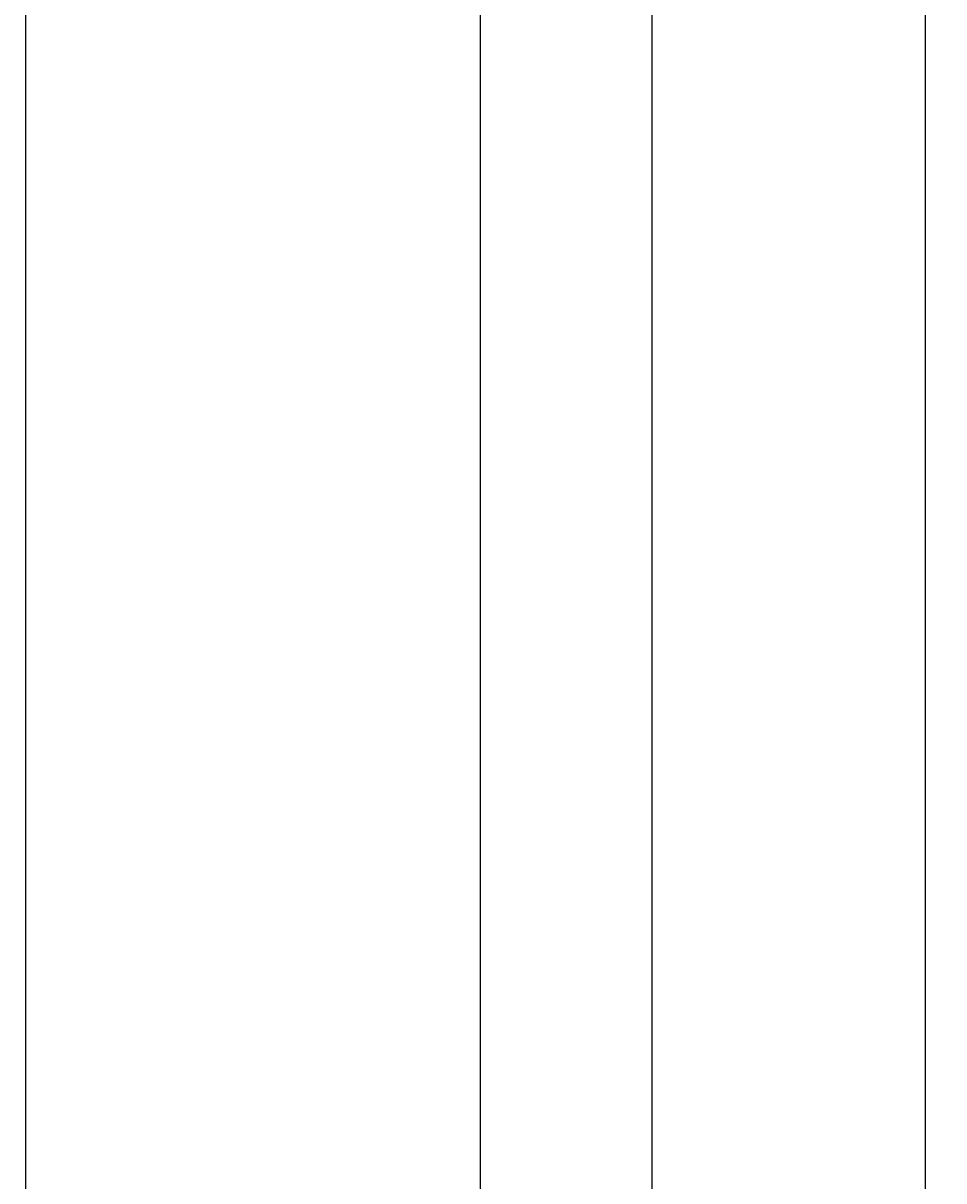
# Model space of a CAD drawing. Units: inches. Extents: x 2231 to 2461, y 2045 to 2455.
# Tile 83 of 95: x 2384 to 2409, y 2352 to 2383. Entities that reach past the tile are written whole.
import ezdxf

# ---------------------------------------------------------------- set-up
doc = ezdxf.new("R2010")
doc.units = ezdxf.units.IN
doc.layers.add('A-ANNO-DIMS', color=2, linetype='Continuous', lineweight=18)
doc.styles.get("Standard").update_dxf_attribs({"font": 'arial.ttf'})
doc.dimstyles.get("Standard").update_dxf_attribs({"dimtxt": 0.18, "dimasz": 0.18, "dimexe": 0.18, "dimexo": 0.0625, "dimgap": 0.09, "dimtad": 0, "dimtih": 1, "dimtoh": 1, "dimdec": 4, "dimzin": 0, "dimdsep": 46, "dimtxsty": 'Standard', "dimcen": 0.09, "dimadec": 0, "dimazin": 0, "dimtfac": 1, "dimtdec": 4, "dimtofl": 0, "dimtmove": 0, "dimatfit": 3, "dimfxl": 1, "dimtolj": 1, "dimtzin": 0, "dimarcsym": 0})

# ---------------------------------------------------------------- blocks, each defined once
blk = doc.blocks.new('*D42')
at = {"layer": 'A-ANNO-DIMS', "color": 0, "lineweight": -2, "transparency": 16777216}
for p, q in [((2396.794, 2286.895), (2396.794, 2454.645)), ((2432.794, 2286.895), (2432.794, 2454.645)), ((2396.974, 2454.465), (2414.575, 2454.465)), ((2432.614, 2454.465), (2415.012, 2454.465))]:
    blk.add_line(p, q, dxfattribs=at)
at = {"layer": 'A-ANNO-DIMS', "color": 0, "transparency": 16777216}
for points in [[(2396.974, 2454.495), (2396.974, 2454.435), (2396.794, 2454.465)], [(2432.614, 2454.495), (2432.614, 2454.435), (2432.794, 2454.465)]]:
    blk.add_solid(points, dxfattribs=at)
at = {"layer": 'Defpoints', "color": 0, "transparency": 16777216}
for p in [(2432.794, 2454.465), (2396.794, 2286.833), (2432.794, 2286.833)]:
    blk.add_point(p, dxfattribs=at)
at = {"layer": 'A-ANNO-DIMS', "color": 0, "transparency": 16777216, "insert": (2414.794, 2454.465), "char_height": 0.18, "attachment_point": 5}
blk.add_mtext('\\A1;36', dxfattribs=at)
blk = doc.blocks.new('*D59')
at = {"layer": 'A-ANNO-DIMS', "color": 0, "lineweight": -2, "transparency": 16777216}
for p, q in [((2408.794, 2182.895), (2408.794, 2454.645)), ((2432.794, 2182.895), (2432.794, 2454.645)), ((2408.974, 2454.465), (2420.573, 2454.465)), ((2432.614, 2454.465), (2421.014, 2454.465))]:
    blk.add_line(p, q, dxfattribs=at)
at = {"layer": 'A-ANNO-DIMS', "color": 0, "transparency": 16777216}
for points in [[(2408.974, 2454.495), (2408.974, 2454.435), (2408.794, 2454.465)], [(2432.614, 2454.495), (2432.614, 2454.435), (2432.794, 2454.465)]]:
    blk.add_solid(points, dxfattribs=at)
at = {"layer": 'Defpoints', "color": 0, "transparency": 16777216}
for p in [(2432.794, 2454.465), (2408.794, 2182.833), (2432.794, 2182.833)]:
    blk.add_point(p, dxfattribs=at)
at = {"layer": 'A-ANNO-DIMS', "color": 0, "transparency": 16777216, "insert": (2420.794, 2454.465), "char_height": 0.18, "attachment_point": 5}
blk.add_mtext('\\A1;24', dxfattribs=at)
blk = doc.blocks.new('*D66')
at = {"layer": 'A-ANNO-DIMS', "color": 0, "lineweight": -2, "transparency": 16777216}
for p, q in [((2348.189, 2096.895), (2348.189, 2454.645)), ((2408.794, 2096.895), (2408.794, 2454.645)), ((2348.369, 2454.465), (2378.167, 2454.465)), ((2408.614, 2454.465), (2378.815, 2454.465))]:
    blk.add_line(p, q, dxfattribs=at)
at = {"layer": 'A-ANNO-DIMS', "color": 0, "transparency": 16777216}
for points in [[(2348.369, 2454.495), (2348.369, 2454.435), (2348.189, 2454.465)], [(2408.614, 2454.495), (2408.614, 2454.435), (2408.794, 2454.465)]]:
    blk.add_solid(points, dxfattribs=at)
at = {"layer": 'Defpoints', "color": 0, "transparency": 16777216}
for p in [(2408.794, 2454.465), (2348.189, 2096.833), (2408.794, 2096.833)]:
    blk.add_point(p, dxfattribs=at)
at = {"layer": 'A-ANNO-DIMS', "color": 0, "transparency": 16777216, "insert": (2378.491, 2454.465), "char_height": 0.18, "attachment_point": 5}
blk.add_mtext('\\A1;60.6', dxfattribs=at)
blk = doc.blocks.new('*D71')
at = {"layer": 'A-ANNO-DIMS', "color": 0, "lineweight": -2, "transparency": 16777216}
for p, q in [((2401.422, 2092.979), (2401.422, 2454.645)), ((2408.794, 2096.895), (2408.794, 2454.645)), ((2401.602, 2454.465), (2404.732, 2454.465)), ((2408.614, 2454.465), (2405.483, 2454.465))]:
    blk.add_line(p, q, dxfattribs=at)
at = {"layer": 'A-ANNO-DIMS', "color": 0, "transparency": 16777216}
for points in [[(2401.602, 2454.495), (2401.602, 2454.435), (2401.422, 2454.465)], [(2408.614, 2454.495), (2408.614, 2454.435), (2408.794, 2454.465)]]:
    blk.add_solid(points, dxfattribs=at)
at = {"layer": 'Defpoints', "color": 0, "transparency": 16777216}
for p in [(2408.794, 2454.465), (2408.794, 2096.833), (2401.422, 2092.917)]:
    blk.add_point(p, dxfattribs=at)
at = {"layer": 'A-ANNO-DIMS', "color": 0, "transparency": 16777216, "insert": (2405.108, 2454.465), "char_height": 0.18, "attachment_point": 5}
blk.add_mtext('\\A1;7.371', dxfattribs=at)
blk = doc.blocks.new('*D72')
at = {"layer": 'A-ANNO-DIMS', "color": 0, "lineweight": -2, "transparency": 16777216}
for p, q in [((2384.543, 2145.12), (2384.543, 2454.645)), ((2408.794, 2150.677), (2408.794, 2454.645)), ((2384.723, 2454.465), (2396.272, 2454.465)), ((2408.614, 2454.465), (2397.064, 2454.465))]:
    blk.add_line(p, q, dxfattribs=at)
at = {"layer": 'A-ANNO-DIMS', "color": 0, "transparency": 16777216}
for points in [[(2384.723, 2454.495), (2384.723, 2454.435), (2384.543, 2454.465)], [(2408.614, 2454.495), (2408.614, 2454.435), (2408.794, 2454.465)]]:
    blk.add_solid(points, dxfattribs=at)
at = {"layer": 'Defpoints', "color": 0, "transparency": 16777216}
for p in [(2408.794, 2454.465), (2408.794, 2150.615), (2384.543, 2145.058)]:
    blk.add_point(p, dxfattribs=at)
at = {"layer": 'A-ANNO-DIMS', "color": 0, "transparency": 16777216, "insert": (2396.668, 2454.465), "char_height": 0.18, "attachment_point": 5}
blk.add_mtext('\\A1;24.25', dxfattribs=at)

msp = doc.modelspace()

# ---------------------------------------------------------------- dimensions: what is measured, and where the dimension line sits
at = {"layer": 'A-ANNO-DIMS'}
for base, p1, p2, override, picture, middle in [((2408.7935, 2454.4653), (2348.1888, 2096.8328), (2408.7935, 2096.8328), {"dimdec": 1, "dimlfac": 1, "dimrnd": 0, "dimzin": 0, "dimdsep": 46, "dimlunit": 2}, '*D66', (2378.4912, 2454.4653)), ((2408.7935, 2454.4653), (2384.5428, 2145.0576), (2408.7935, 2150.6145), {"dimdec": 2, "dimlfac": 1, "dimrnd": 0, "dimzin": 0, "dimdsep": 46, "dimlunit": 2}, '*D72', (2396.6682, 2454.4653)), ((2432.7935, 2454.4653), (2396.7935, 2286.8328), (2432.7935, 2286.8328), {"dimdec": 0, "dimlfac": 1, "dimrnd": 0, "dimzin": 0, "dimdsep": 46, "dimlunit": 2}, '*D42', (2414.7935, 2454.4653)), ((2408.7935, 2454.4653), (2401.4221, 2092.9167), (2408.7935, 2096.8328), {"dimdec": 3, "dimlfac": 1, "dimrnd": 0, "dimzin": 0, "dimdsep": 46, "dimlunit": 2}, '*D71', (2405.1078, 2454.4653)), ((2432.7935, 2454.4653), (2408.7935, 2182.8328), (2432.7935, 2182.8328), {"dimdec": 0, "dimlfac": 1, "dimrnd": 0, "dimzin": 0, "dimdsep": 46, "dimlunit": 2}, '*D59', (2420.7935, 2454.4653))]:
    dim = msp.add_linear_dim(base=base, p1=p1, p2=p2, dimstyle='Standard', override=override, dxfattribs=at)
    dim.commit()
    dim.dimension.update_dxf_attribs({"geometry": picture, "text_midpoint": middle})

doc.saveas('drawing.dxf')
